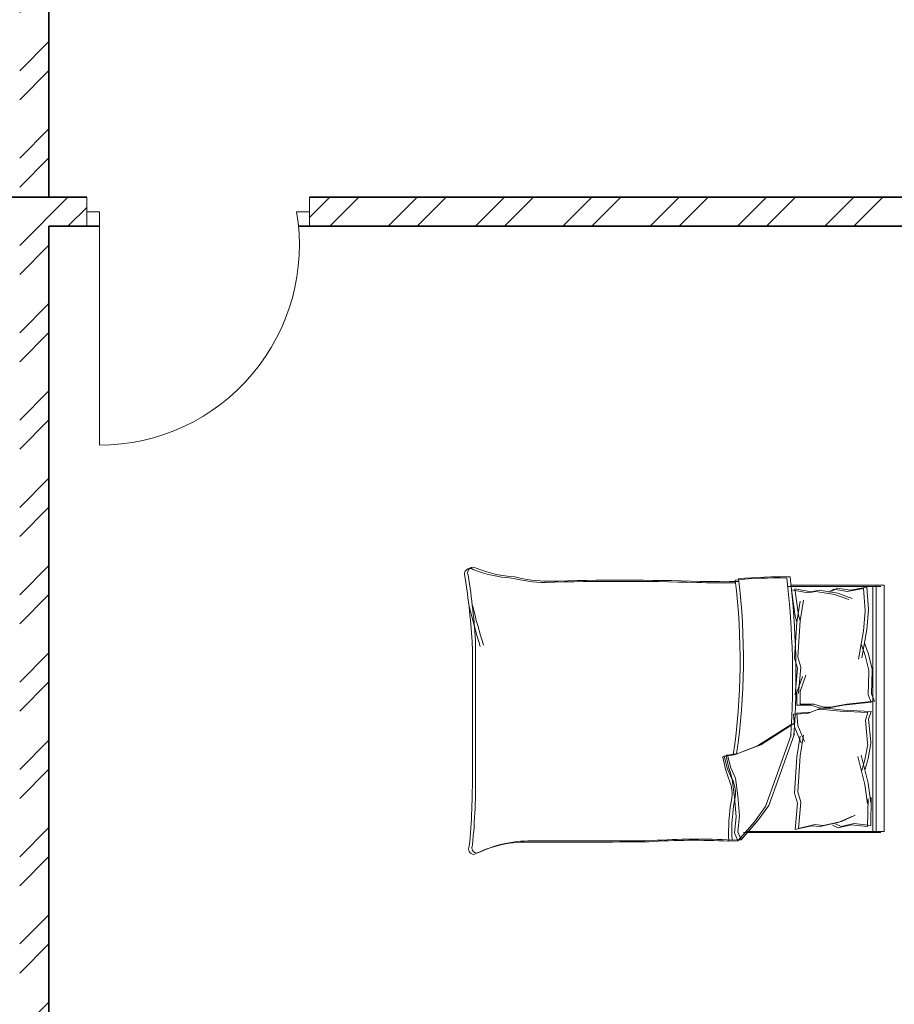
# Model space of a CAD drawing. Units: inches. Extents: x 1962 to 2771, y 1245 to 2660.
# Tile 9 of 114: x 2371 to 2506, y 1527 to 1679. Entities that reach past the tile are written whole.
import ezdxf

# ---------------------------------------------------------------- set-up
doc = ezdxf.new("R2010")
doc.units = ezdxf.units.IN
for name, color, linetype, lineweight in [('A-DOOR', 3, 'Continuous', 18), ('A-FURN', 8, 'Continuous', 13), ('A-WALL', 7, 'Continuous', 35), ('A-WALL-PATT', 252, 'Continuous', 13)]:
    doc.layers.add(name, color=color, linetype=linetype, lineweight=lineweight)

# ---------------------------------------------------------------- blocks, each defined once
blk = doc.blocks.new('BED-PLAN')
for p, q in [((22.05, 42.03), (19.47, 39.08)), ((22.05, 42.02), (19.47, 39.08)), ((22.56, 42.21), (19.98, 39.26)), ((22.56, 42.21), (19.98, 39.26)), ((23.44, 42.09), (22.05, 42.03, 3.08)), ((23.44, 42.09), (22.05, 42.02, 3.08)), ((22.55, 40.8), (22.05, 42.03)), ((22.55, 40.8), (22.05, 42.02)), ((23.95, 42.27), (22.56, 42.21, 3.08)), ((23.95, 42.27), (22.56, 42.21, 3.08)), ((23.06, 40.98), (22.56, 42.21)), ((23.06, 40.98), (22.56, 42.21)), ((0, 40.75), (21.15, 40.75)), ((0, 40.75), (21.15, 40.75)), ((0, 2.76), (0, 40.75)), ((0.51, 40.93), (21.66, 40.93)), ((0.51, 40.93), (21.66, 40.93)), ((1.22, 2.76), (1.22, 40.75)), ((1.22, 2.76), (1.22, 40.75)), ((1.73, 2.95), (1.73, 40.93)), ((1.73, 2.95), (1.73, 40.93)), ((2.03, 39.83), (1.96, 35.54)), ((2.03, 39.83), (1.96, 35.54)), ((2.03, 39.83), (4.58, 39.53)), ((2.03, 39.83), (4.58, 39.53)), ((2.54, 40.02), (2.46, 35.72)), ((2.54, 40.02), (2.46, 35.72)), ((2.54, 40.02), (5.09, 39.72)), ((2.54, 40.02), (5.09, 39.72)), ((4.58, 39.53), (6.63, 40.01)), ((4.58, 39.53), (6.63, 40.01)), ((5.09, 39.72), (7.14, 40.19)), ((5.09, 39.72), (7.14, 40.19)), ((9.4, 39.83), (6.56, 39.2)), ((9.4, 39.83), (6.56, 39.2)), ((6.63, 40.01), (7.46, 39.6)), ((6.63, 40.01), (7.46, 39.6)), ((9.91, 40.02), (7.07, 39.38)), ((9.91, 40.02), (7.07, 39.38)), ((7.14, 40.19), (7.97, 39.78)), ((7.14, 40.19), (7.97, 39.78)), ((10.68, 39.68), (9.4, 39.83)), ((10.68, 39.68), (9.4, 39.83)), ((11.19, 39.87), (9.91, 40.02)), ((11.19, 39.87), (9.91, 40.02)), ((13.17, 40.3), (10.68, 39.68)), ((13.17, 40.3), (10.68, 39.68)), ((13.68, 40.48), (11.19, 39.87)), ((13.68, 40.48), (11.19, 39.87)), ((12.85, 36.22), (13.17, 40.3)), ((12.85, 36.22), (13.17, 40.3)), ((13.36, 36.4), (13.68, 40.48)), ((13.36, 36.4), (13.68, 40.48)), ((22.3, 38.34), (22.55, 40.8)), ((22.3, 38.34), (22.55, 40.8)), ((22.81, 38.52), (23.06, 40.98)), ((22.81, 38.52), (23.06, 40.98)), ((6.56, 39.2), (4.43, 38.26)), ((6.56, 39.2), (4.43, 38.26)), ((7.07, 39.38), (4.94, 38.44)), ((7.07, 39.38), (4.94, 38.44)), ((19.47, 39.08), (17.75, 36.74)), ((19.47, 39.08), (17.75, 36.74)), ((19.98, 39.26), (18.26, 36.92)), ((19.98, 39.26), (18.26, 36.92)), ((22.55, 35.26), (22.3, 38.34)), ((22.55, 35.26), (22.3, 38.34)), ((23.06, 35.45), (22.81, 38.52)), ((23.06, 35.44), (22.81, 38.52)), ((2.46, 35.72), (2.53, 36.52)), ((2.46, 35.72), (2.53, 36.52)), ((2.53, 36.52), (2.95, 33.5)), ((2.53, 36.52), (2.95, 33.5)), ((17.75, 36.74), (16.15, 32.31)), ((17.75, 36.74), (16.15, 32.31)), ((18.26, 36.92), (16.66, 32.49)), ((18.26, 36.92), (16.66, 32.49)), ((1.96, 35.54), (2.02, 36.34)), ((1.96, 35.54), (2.02, 36.34)), ((2.02, 36.34), (2.44, 33.32)), ((2.02, 36.34), (2.44, 33.32)), ((13.3, 34.66), (12.85, 36.22)), ((13.3, 34.66), (12.85, 36.22)), ((13.8, 34.84), (13.36, 36.4)), ((13.8, 34.84), (13.36, 36.4)), ((22.92, 32.56), (22.55, 35.26)), ((22.92, 32.55), (22.55, 35.26)), ((23.42, 32.74), (23.06, 35.45)), ((23.42, 32.74), (23.06, 35.44)), ((2.95, 33.5), (4.02, 29.19)), ((2.95, 33.5), (4.02, 29.19)), ((12.95, 29.09), (13.3, 34.66)), ((12.95, 29.09), (13.3, 34.66)), ((13.46, 29.27), (13.8, 34.84)), ((13.46, 29.27), (13.8, 34.84)), ((2.44, 33.32), (3.52, 29.01)), ((2.44, 33.32), (3.52, 29.01)), ((16.15, 32.31), (13.82, 25.68)), ((16.15, 32.31), (13.82, 25.68)), ((16.66, 32.49), (14.33, 25.86)), ((16.66, 32.49), (14.33, 25.86)), ((23.65, 30.95), (22.92, 32.56)), ((23.65, 30.95), (22.92, 32.55)), ((24.16, 31.14), (23.42, 32.74)), ((24.16, 31.14), (23.42, 32.74)), ((2.92, 31.16), (2.45, 29.52)), ((2.92, 31.16), (2.45, 29.52)), ((3.43, 31.34), (2.96, 29.7)), ((3.43, 31.34), (2.96, 29.7)), ((24.15, 28.99), (23.65, 30.95)), ((24.15, 28.98), (23.65, 30.95)), ((24.65, 29.17), (24.16, 31.14)), ((24.65, 29.17), (24.16, 31.14)), ((62.99, 11.98), (62.99, 31.54)), ((62.99, 11.97), (62.99, 31.54)), ((63.5, 12.16), (63.5, 31.72)), ((63.5, 12.16), (63.5, 31.72)), ((2.45, 29.52), (2.02, 27.19)), ((2.45, 29.52), (2.02, 27.19)), ((2.96, 29.7), (2.52, 27.37)), ((2.96, 29.7), (2.52, 27.37)), ((12.42, 25.89), (12.95, 29.09)), ((12.42, 25.89), (12.95, 29.09)), ((12.93, 26.07), (13.46, 29.27)), ((12.93, 26.07), (13.46, 29.27)), ((19.49, 27.57), (23.06, 28.92)), ((19.49, 27.57), (23.06, 28.92)), ((22.55, 28.74), (24.15, 28.99)), ((22.55, 28.74), (24.15, 28.98)), ((23.06, 28.92), (24.65, 29.17)), ((23.06, 28.92), (24.65, 29.17)), ((2.52, 27.37), (2.54, 27.12)), ((2.52, 27.37), (2.54, 27.12)), ((13.82, 24.05), (18.98, 27.38)), ((13.82, 24.05), (18.98, 27.38)), ((14.33, 24.24), (19.49, 27.57)), ((14.33, 24.24), (19.49, 27.57)), ((18.98, 27.38), (22.55, 28.74)), ((18.98, 27.38), (22.55, 28.74)), ((2.02, 27.19), (2.03, 26.94)), ((2.02, 27.19), (2.03, 26.93)), ((2.03, 26.94), (2.37, 23.42)), ((2.03, 26.93), (2.37, 23.42)), ((2.54, 27.12), (2.88, 23.6)), ((2.54, 27.12), (2.88, 23.6)), ((13.31, 24.44), (12.28, 26.89)), ((13.31, 24.44), (12.28, 26.88)), ((13.81, 24.63), (12.79, 27.07)), ((13.81, 24.63), (12.79, 27.07)), ((13.43, 22.49), (13.31, 24.44)), ((13.43, 22.49), (13.31, 24.44)), ((13.94, 22.68), (13.81, 24.63)), ((13.94, 22.68), (13.81, 24.63)), ((2.37, 23.42), (1.98, 22.24)), ((2.37, 23.42), (1.98, 22.24)), ((2.88, 23.6), (2.49, 22.42)), ((2.88, 23.6), (2.49, 22.42)), ((1.98, 22.24), (6.25, 22.05)), ((1.98, 22.24), (6.25, 22.05)), ((1.99, 20.84), (6.25, 21.3)), ((1.99, 20.84), (6.25, 21.3)), ((2.49, 22.42), (6.76, 22.23)), ((2.49, 22.42), (6.76, 22.23)), ((5.74, 21.11), (8.27, 21.57)), ((5.74, 21.11), (8.27, 21.57)), ((6.25, 22.05), (8.81, 21.75)), ((6.25, 22.05), (8.81, 21.75)), ((6.25, 21.3), (8.78, 21.76)), ((6.25, 21.3), (8.78, 21.76)), ((6.76, 22.23), (9.31, 21.93)), ((6.76, 22.23), (9.31, 21.93)), ((8.27, 21.57), (9.3, 21.57)), ((8.27, 21.57), (9.3, 21.57)), ((8.78, 21.76), (9.81, 21.76)), ((8.78, 21.76), (9.81, 21.76)), ((8.81, 21.75), (9.84, 21.81)), ((8.81, 21.75), (9.84, 21.81)), ((9.3, 21.57), (10.8, 21.11)), ((9.3, 21.57), (10.8, 21.11)), ((9.31, 21.93), (10.35, 21.99)), ((9.31, 21.93), (10.35, 21.99)), ((9.81, 21.76), (11.3, 21.3)), ((9.81, 21.76), (11.3, 21.3)), ((9.84, 21.81), (11.3, 22.36)), ((9.84, 21.81), (11.3, 22.36)), ((10.35, 21.99), (11.81, 22.54)), ((10.35, 21.99), (11.81, 22.54)), ((11.3, 22.36), (13.43, 22.49)), ((11.3, 22.36), (13.43, 22.49)), ((11.3, 21.3), (13.44, 21.3)), ((11.3, 21.3), (13.44, 21.3)), ((11.81, 22.54), (13.94, 22.68)), ((11.81, 22.54), (13.94, 22.68)), ((13.44, 21.3), (13.44, 19.34)), ((13.44, 21.3), (13.44, 19.34)), ((1.49, 20.65), (5.74, 21.11)), ((1.49, 20.65), (5.74, 21.11)), ((1.95, 19.51), (1.49, 20.65)), ((1.95, 19.51), (1.49, 20.65)), ((2.45, 19.69), (1.99, 20.84)), ((2.45, 19.69), (1.99, 20.84)), ((10.8, 21.11), (12.93, 21.11)), ((10.8, 21.11), (12.93, 21.11)), ((12.93, 21.11), (12.93, 19.16)), ((12.93, 21.11), (12.93, 19.16)), ((1.83, 15.97), (1.95, 19.51)), ((1.83, 15.97), (1.95, 19.51)), ((2.34, 16.15), (2.45, 19.69)), ((2.34, 16.15), (2.45, 19.69)), ((12.93, 19.16), (12.06, 16.66)), ((12.93, 19.16), (12.06, 16.66)), ((13.44, 19.34), (12.57, 16.84)), ((13.44, 19.34), (12.57, 16.84)), ((12.85, 15.41), (13.17, 19.49)), ((12.85, 15.41), (13.17, 19.49)), ((13.36, 15.59), (13.68, 19.67)), ((13.36, 15.59), (13.68, 19.67)), ((1.83, 15.72), (1.83, 15.97)), ((1.83, 15.72), (1.83, 15.97)), ((2.41, 13.42), (1.83, 15.72)), ((2.41, 13.42), (1.83, 15.72)), ((2.34, 15.9), (2.34, 16.15)), ((2.34, 15.9), (2.34, 16.15)), ((2.91, 13.6), (2.34, 15.9)), ((2.91, 13.6), (2.34, 15.9)), ((13.3, 13.85), (12.85, 15.41)), ((13.3, 13.85), (12.85, 15.41)), ((13.8, 14.03), (13.36, 15.59)), ((13.8, 14.03), (13.36, 15.59)), ((2.64, 9.63), (3.44, 13.99)), ((2.64, 9.63), (3.44, 13.99)), ((3.14, 9.81), (3.95, 14.17)), ((3.14, 9.81), (3.95, 14.17)), ((12.95, 8.28), (13.3, 13.85)), ((12.95, 8.28), (13.3, 13.85)), ((13.46, 8.46), (13.8, 14.03)), ((13.46, 8.46), (13.8, 14.03)), ((2.98, 11.81), (2.41, 13.42)), ((2.98, 11.81), (2.41, 13.42)), ((3.49, 11.99), (2.91, 13.6)), ((3.49, 11.99), (2.91, 13.6)), ((2.41, 6.59), (2.64, 9.63)), ((2.41, 6.59), (2.64, 9.63)), ((2.91, 6.77), (3.14, 9.81)), ((2.91, 6.77), (3.14, 9.81)), ((12.42, 5.07), (12.95, 8.28)), ((12.42, 5.07), (12.95, 8.28)), ((12.93, 5.26), (13.46, 8.46)), ((12.93, 5.26), (13.46, 8.46)), ((12.95, 8.28), (13.21, 7.38)), ((12.95, 8.28), (13.21, 7.38)), ((13.46, 8.46), (13.72, 7.56)), ((13.46, 8.46), (13.72, 7.56)), ((2.39, 6.5), (2.41, 6.59)), ((2.39, 6.5), (2.41, 6.59)), ((2.65, 3.1), (2.39, 6.5)), ((2.65, 3.1), (2.39, 6.5)), ((2.9, 6.68), (2.91, 6.77)), ((2.9, 6.68), (2.91, 6.77)), ((3.16, 3.28), (2.9, 6.68)), ((3.16, 3.28), (2.9, 6.68)), ((13.21, 7.38), (13.78, 3.33)), ((13.21, 7.38), (13.78, 3.33)), ((13.72, 7.56), (14.29, 3.51)), ((13.72, 7.56), (14.29, 3.51)), ((7.12, 4.02), (4.93, 4.82)), ((7.12, 4.02), (4.93, 4.82)), ((7.63, 4.2), (5.44, 5)), ((7.63, 4.2), (5.44, 5)), ((2.64, 3.1), (5.16, 3.56)), ((2.64, 3.1), (5.16, 3.56)), ((3.14, 3.28), (5.67, 3.74)), ((3.14, 3.28), (5.67, 3.74)), ((5.16, 3.56), (7.23, 3.21)), ((5.16, 3.56), (7.23, 3.21)), ((5.67, 3.74), (7.74, 3.39)), ((5.67, 3.74), (7.74, 3.39)), ((9.99, 3.56), (7.12, 4.02)), ((9.99, 3.56), (7.12, 4.02)), ((7.23, 3.21), (8.04, 3.67)), ((7.23, 3.21), (8.04, 3.67)), ((10.5, 3.74), (7.63, 4.2)), ((10.5, 3.74), (7.63, 4.2)), ((7.74, 3.39), (8.55, 3.85)), ((7.74, 3.39), (8.55, 3.85)), ((11.26, 3.79), (9.99, 3.56)), ((11.26, 3.79), (9.99, 3.56)), ((11.76, 3.97), (10.5, 3.74)), ((11.76, 3.97), (10.5, 3.74)), ((13.78, 3.33), (11.26, 3.79)), ((13.78, 3.33), (11.26, 3.79)), ((14.29, 3.51), (11.76, 3.97)), ((14.29, 3.51), (11.76, 3.97)), ((14.4, 2.76), (0, 2.76)), ((14.4, 2.76), (0, 2.76)), ((14.9, 2.95), (0.51, 2.95)), ((14.9, 2.95), (0.51, 2.95))]:
    blk.add_line(p, q)
for centre, radius, start, end in [((54.58, 60.54), 18.33, 267.4714, 296.4681), ((54.58, 60.54), 18.33, 267.4714, 296.4681), ((55.09, 60.72), 18.33, 267.4714, 296.4681), ((55.09, 60.72), 18.33, 267.4714, 296.4681), ((62.69, 43.25), 0.876, 332.6588, 86.02), ((62.69, 43.25), 0.876, 332.6588, 86.02), ((63.2, 43.43), 0.876, 332.6588, 86.02), ((63.2, 43.43), 0.876, 332.6588, 86.02), ((168.74, 32.71), 105.75, 174.4998, 180.6351), ((168.74, 32.71), 105.75, 174.4998, 180.6351), ((169.24, 32.89), 105.75, 174.4998, 180.6351), ((169.24, 32.89), 105.75, 174.4998, 180.6351), ((-5.29, 40.8), 28.76, 349.8763, 2.5657), ((-5.29, 40.8), 28.76, 349.8763, 2.5657), ((28.87, 144.88), 102.94, 266.9791, 273.8365), ((28.87, 144.88), 102.94, 266.9791, 273.8365), ((-4.78, 40.98), 28.76, 349.8763, 2.5657), ((-4.78, 40.98), 28.76, 349.8763, 2.5657), ((29.37, 145.06), 102.94, 266.9791, 273.8365), ((29.37, 145.06), 102.94, 266.9791, 273.8365), ((53.91, -3583.94), 3626.16, 90.00217, 90.28689), ((53.91, -3583.94), 3626.16, 90.00217, 90.28689), ((54.42, -3583.75), 3626.16, 90.00217, 90.28689), ((54.42, -3583.75), 3626.16, 90.00217, 90.28689), ((27.87, 34.77), 4.95, 168.6608, 203.7384), ((27.87, 34.77), 4.95, 168.6608, 203.7384), ((28.38, 34.95), 4.95, 168.6608, 203.7384), ((28.38, 34.95), 4.95, 168.6608, 203.7384), ((1.18, 24.77), 23.57, 10.6617, 19.8806), ((1.18, 24.76), 23.57, 10.6617, 19.8806), ((1.69, 24.95), 23.57, 10.6617, 19.8806), ((1.69, 24.95), 23.57, 10.6617, 19.8806), ((124.76, 14.3), 102.56, 171.7845, 186.9006), ((124.76, 14.3), 102.56, 171.7845, 186.9006), ((24.2, 29.12), 0.147, 250.2464, 1.1377), ((24.2, 29.12), 0.147, 250.2464, 1.1377), ((24.7, 29.3), 0.147, 250.2464, 1.1377), ((24.7, 29.3), 0.147, 250.2464, 1.1377), ((124.25, 14.12), 102.56, 171.7845, 186.9006), ((124.25, 14.11), 102.56, 171.7845, 186.9006), ((144.71, 16.98), 131.13, 176.0865, 186.7821), ((144.71, 16.98), 131.13, 176.0865, 186.7821), ((145.22, 17.16), 131.13, 176.0865, 186.7821), ((145.22, 17.16), 131.13, 176.0865, 186.7821), ((-18.34, -13.51), 84.62, 13.3832, 17.7053), ((-18.34, -13.51), 84.62, 13.3832, 17.7053), ((160.15, 17.21), 96.78, 182.9958, 189.4091), ((160.15, 17.21), 96.78, 182.9958, 189.4091), ((-18.85, -13.69), 84.62, 13.3832, 17.7053), ((-18.85, -13.69), 84.62, 13.3832, 17.7053), ((159.64, 17.03), 96.78, 182.9958, 189.4091), ((159.64, 17.03), 96.78, 182.9958, 189.4091), ((15.97, 67.7), 66.22, 268.7218, 275.604), ((15.97, 67.7), 66.22, 268.7218, 275.604), ((16.48, 67.88), 66.22, 268.7218, 275.604), ((16.48, 67.88), 66.22, 268.7218, 275.604), ((24.78, -132.99), 135.22, 88.4762, 91.0082), ((24.78, -132.99), 135.22, 88.4762, 91.0082), ((25.29, -132.81), 135.22, 88.4762, 91.0082), ((25.29, -132.81), 135.22, 88.4762, 91.0082), ((40.23, 385.38), 383.38, 268.2277, 271.7185), ((40.23, 385.38), 383.38, 268.2277, 271.7185), ((40.74, 385.56), 383.38, 268.2277, 271.7185), ((40.74, 385.56), 383.38, 268.2277, 271.7185), ((51.28, -21.38), 23.56, 76.0648, 88.9113), ((51.28, -21.38), 23.56, 76.0648, 88.9113), ((51.79, -21.2), 23.56, 76.0648, 88.9113), ((51.79, -21.2), 23.56, 76.0648, 88.9113), ((56.37, -17.03), 18.73, 67.9751, 86.652), ((56.37, -17.03), 18.73, 67.9751, 86.652), ((55.86, -17.22), 18.73, 67.9751, 86.652), ((55.86, -17.22), 18.73, 67.9751, 86.652), ((63.37, 0.87), 0.866, 236.1736, 23.4781), ((63.37, 0.87), 0.866, 236.1736, 23.4781), ((63.87, 1.05), 0.866, 236.1736, 23.4781), ((63.87, 1.05), 0.866, 236.1736, 23.4781)]:
    blk.add_arc(centre, radius, start, end)

msp = doc.modelspace()

# ---------------------------------------------------------------- hatches: boundary and pattern name
at = {"layer": 'A-WALL-PATT'}
h = msp.add_hatch(dxfattribs=at)
h.set_pattern_fill('ANSI32', color=256)
h.paths.add_polyline_path([(2090.8074, 2467.3437), (2141.6481, 2467.3437), (2141.6481, 2469.5937), (2141.6481, 2471.8437), (2086.3074, 2471.8437), (2086.3074, 2422.5333), (2090.8074, 2422.5333)])
h.paths.add_polyline_path([(2282.7664, 2471.8437), (2204.8982, 2471.8437), (2204.8982, 2467.3437), (2234.8074, 2467.3437), (2234.8074, 2311.3437), (2228.7492, 2311.3437), (2228.7492, 2306.8437), (2234.8074, 2306.8437), (2331.9227, 2306.8437), (2331.9227, 2309.0937), (2331.9227, 2311.3437), (2239.3074, 2311.3437), (2239.3074, 2467.3437), (2282.7664, 2467.3437), (2282.7664, 2469.5937)])
h.paths.add_polyline_path([(2471.4531, 2519.8437), (2552.011, 2519.8437), (2564.3996, 2519.8437), (2564.3996, 2511.1389), (2568.8996, 2511.1389), (2568.8996, 2524.3437), (2466.9531, 2524.3437), (2466.9531, 2471.8437), (2450.0749, 2471.8437), (2446.4672, 2471.8437), (2446.4672, 2467.3437), (2450.0749, 2467.3437), (2475.9988, 2467.3437), (2475.9988, 2469.5937), (2475.9988, 2471.8437), (2471.4531, 2471.8437)])
h.paths.add_polyline_path([(2575.2231, 2469.5937), (2575.2231, 2471.8437), (2568.8996, 2471.8437), (2568.8996, 2487.1389), (2564.3996, 2487.1389), (2564.3996, 2471.8437), (2556.511, 2471.8437), (2499.2904, 2471.8437), (2499.2904, 2467.3437), (2507.8074, 2467.3437), (2507.8074, 2311.3437), (2414.863, 2311.3437), (2414.863, 2306.8437), (2512.3074, 2306.8437), (2517.0114, 2306.8437), (2517.0114, 2309.0937), (2517.0114, 2311.3437), (2512.3074, 2311.3437), (2512.3074, 2467.3437), (2575.2231, 2467.3437)])
h.paths.add_polyline_path([(2660.8074, 2471.8437), (2600.9602, 2471.8437), (2600.9602, 2467.3437), (2656.3074, 2467.3437), (2656.3074, 2432.5704), (2660.8074, 2432.5704)])
h.paths.add_polyline_path([(2660.8074, 2372.5704), (2656.3074, 2372.5704), (2656.3074, 2311.3437), (2600.276, 2311.3437), (2600.276, 2309.0937), (2600.276, 2306.8437), (2656.3074, 2306.8437), (2656.3074, 2296.2593), (2660.8074, 2296.2593)])
h.paths.add_polyline_path([(2572.3074, 2306.8437), (2577.1385, 2306.8437), (2577.1385, 2311.3437), (2551.082, 2311.3437), (2551.082, 2306.8437), (2567.8074, 2306.8437), (2567.8074, 2258.8437), (2540.0574, 2258.8437), (2540.0574, 2256.5937), (2540.0574, 2254.3437), (2567.8074, 2254.3437), (2656.3074, 2254.3437), (2656.3074, 2236.9085), (2660.8074, 2236.9085), (2660.8074, 2272.2593), (2656.3074, 2272.2593), (2656.3074, 2258.8437), (2572.3074, 2258.8437)])
h.paths.add_polyline_path([(2512.3074, 2254.3437), (2518.8716, 2254.3437), (2518.8716, 2256.5937), (2518.8716, 2258.8437), (2507.8074, 2258.8437), (2507.8074, 2177.8437), (2567.8074, 2177.8437), (2567.8074, 2172.9628), (2572.3074, 2172.9628), (2572.3074, 2177.8437), (2656.3074, 2177.8437), (2656.3074, 2166.4846), (2660.8074, 2166.4846), (2660.8074, 2200.9085), (2656.3074, 2200.9085), (2656.3074, 2182.3437), (2512.3074, 2182.3437)])
h.paths.add_polyline_path([(2656.3074, 2129.8437), (2572.3074, 2129.8437), (2572.3074, 2150.3044), (2570.0574, 2150.3044), (2567.8074, 2150.3044), (2567.8074, 2129.8437), (2507.8074, 2129.8437), (2507.8074, 2116.3027), (2510.0574, 2116.3027), (2512.3074, 2116.3027), (2512.3074, 2125.3437), (2567.8074, 2125.3437), (2572.3074, 2125.3437), (2656.3074, 2125.3437)])
h.paths.add_polyline_path([(2090.8074, 2362.5333), (2086.3074, 2362.5333), (2086.3074, 2298.6242), (2090.8074, 2298.6242), (2090.8074, 2306.8437), (2174.8074, 2306.8437), (2174.8074, 2286.4178), (2179.3074, 2286.4178), (2179.3074, 2306.8437), (2192.8641, 2306.8437), (2192.8641, 2309.0937), (2192.8641, 2311.3437), (2090.8074, 2311.3437)])
h.paths.add_polyline_path([(2209.156, 2258.8437), (2179.3074, 2258.8437), (2179.3074, 2263.2236), (2177.0574, 2263.2236), (2174.8074, 2263.2236), (2174.8074, 2258.8437), (2090.8074, 2258.8437), (2090.8074, 2274.6242), (2086.3074, 2274.6242), (2086.3074, 2238.2967), (2088.5574, 2238.2967), (2090.8074, 2238.2967), (2090.8074, 2254.3437), (2209.156, 2254.3437)])
h.paths.add_polyline_path([(2090.8074, 2177.8437), (2234.8074, 2177.8437), (2234.8074, 2173.1428), (2239.3074, 2173.1428), (2239.3074, 2258.8437), (2230.8442, 2258.8437), (2230.8442, 2256.5937), (2230.8442, 2254.3437), (2234.8074, 2254.3437), (2234.8074, 2182.3437), (2090.8074, 2182.3437), (2090.8074, 2202.2967), (2086.3074, 2202.2967), (2086.3074, 2140.0389), (2090.8074, 2140.0389)])
h.paths.add_polyline_path([(2090.8074, 2080.0389), (2086.3074, 2080.0389), (2086.3074, 2033.8437), (2090.8074, 2033.8437)], flags=17)
h.paths.add_polyline_path([(2244.9405, 2033.8437), (2239.3074, 2033.8437), (2239.3074, 2142.0665), (2237.2592, 2142.0665), (2234.8074, 2142.0665), (2234.8074, 2033.8437), (2090.8074, 2033.8437), (2076.5204, 2033.8437), (2072.0204, 2033.8437), (2072.0204, 2000.4493), (2076.5204, 2000.4493), (2076.5204, 2029.3437), (2090.8074, 2029.3437), (2244.9405, 2029.3437), (2244.9405, 2031.5937)])
h.paths.add_polyline_path([(2234.8074, 1933.3437), (2076.5204, 1933.3437), (2076.5204, 1952.4493), (2074.2704, 1952.4493), (2072.0204, 1952.4493), (2072.0204, 1933.3437), (2072.0204, 1928.8437), (2234.8074, 1928.8437)])
h.paths.add_polyline_path([(2090.8074, 1928.8437), (2086.3074, 1928.8437), (2086.3074, 1906.5013), (2090.8074, 1906.5013)])
h.paths.add_polyline_path([(2090.8074, 1846.5013), (2086.3074, 1846.5013), (2086.3074, 1769.9917), (2088.5574, 1769.9917), (2090.8074, 1769.9917), (2090.8074, 1780.3437), (2234.8074, 1780.3437), (2234.8074, 1708.3437), (2230.3764, 1708.3437), (2230.3764, 1703.8437), (2239.3074, 1703.8437), (2239.3074, 1792.6669), (2237.0574, 1792.6669), (2234.8074, 1792.6669), (2234.8074, 1784.8437), (2090.8074, 1784.8437)])
h.paths.add_polyline_path([(2239.3074, 1928.8437), (2244.9405, 1928.8437), (2244.9405, 1931.0937), (2244.9405, 1933.3437), (2234.8074, 1933.3437), (2234.8074, 1928.8437), (2234.8074, 1825.5949), (2239.3074, 1825.5949)])
h.paths.add_polyline_path([(2148.0425, 1649.0937), (2148.0425, 1651.3437), (2090.8074, 1651.3437), (2090.8074, 1646.8437), (2148.0425, 1646.8437)], flags=0)
h.paths.add_polyline_path([(2207.5601, 1708.3437), (2090.8074, 1708.3437), (2090.8074, 1703.8437), (2174.8074, 1703.8437), (2174.8074, 1651.3437), (2170.4457, 1651.3437), (2170.4457, 1646.8437), (2195.9924, 1646.8437), (2195.9924, 1649.0937), (2195.9924, 1651.3437), (2179.3074, 1651.3437), (2179.3074, 1703.8437), (2207.5601, 1703.8437), (2207.5601, 1706.0937)])
h.paths.add_polyline_path([(2090.8074, 1733.9917), (2086.3074, 1733.9917), (2086.3074, 1696.1032), (2088.5574, 1696.1032), (2090.8074, 1696.1032)])
h.paths.add_polyline_path([(2090.8074, 1672.1032), (2086.3074, 1672.1032), (2086.3074, 1600.3335), (2090.8074, 1600.3335)])
h.paths.add_polyline_path([(2090.8074, 1540.3335), (2086.3074, 1540.3335), (2086.3074, 1486.3437), (2139.6766, 1486.3437), (2139.6766, 1490.8437), (2090.8074, 1490.8437)])
h.paths.add_polyline_path([(2302.3876, 1490.8437), (2239.3074, 1490.8437), (2239.3074, 1646.8437), (2335.9994, 1646.8437), (2335.9994, 1651.3437), (2229.884, 1651.3437), (2229.884, 1646.8437), (2234.8074, 1646.8437), (2234.8074, 1490.8437), (2202.7103, 1490.8437), (2202.7103, 1488.5937), (2202.7103, 1486.3437), (2275.0699, 1486.3437), (2275.0699, 1475.772), (2279.5699, 1475.772), (2279.5699, 1486.3437), (2302.3876, 1486.3437)])
h.paths.add_polyline_path([(2279.5699, 1451.772), (2275.0699, 1451.772), (2275.0699, 1438.3437), (2174.8074, 1438.3437), (2174.8074, 1486.3437), (2179.7922, 1486.3437), (2179.7922, 1490.8437), (2163.3585, 1490.8437), (2163.3585, 1488.5937), (2163.3585, 1486.3437), (2170.3074, 1486.3437), (2170.3074, 1433.8437), (2279.5699, 1433.8437)])
h.paths.add_polyline_path([(2427.2363, 1490.8437), (2375.8074, 1490.8437), (2375.8074, 1646.8437), (2381.6401, 1646.8437), (2381.6401, 1651.3437), (2365.887, 1651.3437), (2365.887, 1649.0937), (2365.887, 1646.8437), (2371.3074, 1646.8437), (2371.3074, 1490.8437), (2327.5627, 1490.8437), (2327.5627, 1488.5937), (2327.5627, 1486.3437), (2371.3074, 1486.3437), (2371.3074, 1433.8437), (2375.8074, 1433.8437), (2375.8074, 1486.3437), (2427.2363, 1486.3437)])
h.paths.add_polyline_path([(2512.3074, 1646.8437), (2519.4351, 1646.8437), (2519.4351, 1649.0937), (2519.4351, 1651.3437), (2507.8074, 1651.3437), (2416.0063, 1651.3437), (2416.0063, 1649.0937), (2416.0063, 1646.8437), (2507.8074, 1646.8437), (2507.8074, 1490.8437), (2497.0532, 1490.8437), (2497.0532, 1488.5937), (2497.0532, 1486.3437), (2574.9344, 1486.3437), (2574.9344, 1476.0181), (2579.4344, 1476.0181), (2579.4344, 1486.3437), (2584.4872, 1486.3437), (2584.3074, 1490.8437), (2512.3074, 1490.8437)])
h.paths.add_polyline_path([(2470.5091, 1486.3437), (2473.9767, 1486.3437), (2473.9767, 1490.8437), (2449.6605, 1490.8437), (2449.6605, 1488.5937), (2449.6605, 1486.3437), (2466.0091, 1486.3437), (2466.0091, 1433.8437), (2470.5091, 1433.8437), (2579.4344, 1433.8437), (2579.4344, 1452.0181), (2574.9344, 1452.0181), (2574.9344, 1438.3437), (2554.5091, 1438.3437), (2470.5091, 1438.3437)])
h.paths.add_polyline_path([(2656.3074, 1490.8437), (2611.86, 1490.8437), (2611.86, 1486.3437), (2656.3074, 1486.3437)])
h.paths.add_polyline_path([(2660.8074, 1532.7007), (2658.5574, 1532.7007), (2656.3074, 1532.7007), (2656.3074, 1486.3437), (2660.8074, 1486.3437)])
h.paths.add_polyline_path([(2660.8074, 1664.9663), (2656.3074, 1664.9663), (2656.3074, 1651.3437), (2602.2313, 1651.3437), (2602.2313, 1646.8437), (2656.3074, 1646.8437), (2656.3074, 1592.7007), (2660.8074, 1592.7007)])
h.paths.add_polyline_path([(2660.8074, 1724.5221), (2656.3074, 1724.5221), (2656.3074, 1703.8437), (2542.4725, 1703.8437), (2542.4725, 1699.3437), (2567.8074, 1699.3437), (2567.8074, 1651.3437), (2552.7766, 1651.3437), (2552.7766, 1649.0937), (2552.7766, 1646.8437), (2577.2878, 1646.8437), (2577.2878, 1649.0937), (2577.2878, 1651.3437), (2572.3074, 1651.3437), (2572.3074, 1699.3437), (2656.3074, 1699.3437), (2656.3074, 1688.9663), (2660.8074, 1688.9663)])
h.paths.add_polyline_path([(2660.8074, 1880.6524), (2656.3074, 1880.6524), (2656.3074, 1832.8437), (2512.3074, 1832.8437), (2512.3074, 1837.8959), (2507.8074, 1837.8959), (2507.8074, 1828.3437), (2567.8074, 1828.3437), (2567.8074, 1804.3437), (2572.3074, 1804.3437), (2572.3074, 1828.3437), (2656.3074, 1828.3437), (2656.3074, 1818.6778), (2660.8074, 1818.6778)])
h.paths.add_polyline_path([(2660.8074, 1794.6778), (2656.3074, 1794.6778), (2656.3074, 1780.3437), (2572.3074, 1780.3437), (2572.3074, 1783.0303), (2570.0574, 1783.0303), (2567.8074, 1783.0303), (2567.8074, 1780.3437), (2507.8074, 1780.3437), (2507.8074, 1699.3437), (2517.8858, 1699.3437), (2517.8858, 1701.5937), (2517.8858, 1703.8437), (2512.3074, 1703.8437), (2512.3074, 1775.8437), (2656.3074, 1775.8437), (2656.3074, 1760.5221), (2660.8074, 1760.5221)])
h.paths.add_polyline_path([(2660.8074, 1981.3437), (2660.8074, 2020.2808), (2658.5574, 2020.2808), (2656.3074, 2020.2808), (2656.3074, 1981.3437), (2512.3074, 1981.3437), (2512.3074, 2086.6996), (2507.8074, 2086.6996), (2507.8074, 1981.3437), (2375.8074, 1981.3437), (2375.8074, 1986.8505), (2373.5574, 1986.8505), (2371.3074, 1986.8505), (2371.3074, 1973.2607), (2375.8074, 1973.2607), (2375.8074, 1976.8437), (2507.8074, 1976.8437), (2507.8074, 1865.4281), (2510.0574, 1865.4281), (2512.3074, 1865.4281), (2512.3074, 1976.8437), (2660.8074, 1976.8437)])
h.paths.add_polyline_path([(2375.8074, 1940.297), (2373.5574, 1940.297), (2371.3074, 1940.297), (2371.3074, 1933.3437), (2278.4434, 1933.3437), (2278.4434, 1928.8437), (2371.3074, 1928.8437), (2371.3074, 1651.3437), (2375.8074, 1651.3437)])
h.paths.add_polyline_path([(2660.8074, 1976.8437), (2656.3074, 1976.8437), (2656.3074, 1940.6524), (2660.8074, 1940.6524)], flags=17)
h.paths.add_polyline_path([(2660.8074, 2142.4846), (2656.3074, 2142.4846), (2656.3074, 2080.2808), (2660.8074, 2080.2808)])
h.paths.add_polyline_path([(2381.4189, 2311.3437), (2375.8074, 2311.3437), (2375.8074, 2467.3437), (2424.7242, 2467.3437), (2424.7242, 2469.5937), (2424.7242, 2471.8437), (2375.8074, 2471.8437), (2375.8074, 2524.3437), (2371.3074, 2524.3437), (2371.3074, 2471.8437), (2307.2097, 2471.8437), (2307.2097, 2467.3437), (2371.3074, 2467.3437), (2371.3074, 2311.3437), (2366.8901, 2311.3437), (2366.8901, 2306.8437), (2371.3074, 2306.8437), (2371.3074, 2033.8437), (2279.6589, 2033.8437), (2279.6589, 2029.3437), (2371.3074, 2029.3437), (2371.3074, 2014.2598), (2375.8074, 2014.2598), (2375.8074, 2306.8437), (2381.4189, 2306.8437)])
h.paths.add_polyline_path([(2263.3074, 2524.3437), (2170.3074, 2524.3437), (2170.3074, 2519.8437), (2170.3074, 2471.8437), (2165.0312, 2471.8437), (2165.0312, 2467.3437), (2179.6721, 2467.3437), (2179.6721, 2469.5161), (2179.6721, 2471.8437), (2174.8074, 2471.8437), (2174.8074, 2519.8437), (2258.8074, 2519.8437), (2258.8074, 2511.6436), (2263.3074, 2511.6436)])
h.paths.add_polyline_path([(2245.0232, 1361.4123), (2492.9468, 1361.4123), (2492.9468, 1398.505), (2245.0232, 1398.505)], flags=9)
h.paths.add_polyline_path([(2388.1434, 2086.6936), (2425.0704, 2086.6936), (2425.0704, 2105.3509), (2388.1434, 2105.3509)], flags=9)
h.paths.add_polyline_path([(2404.922, 2242.6744), (2445.7337, 2242.6744), (2445.7337, 2261.3318), (2404.922, 2261.3318)], flags=9)
h.paths.add_polyline_path([(2269.4107, 2156.7935), (2306.3378, 2156.7935), (2306.3378, 2175.4508), (2269.4107, 2175.4508)], flags=9)
h.paths.add_polyline_path([(2269.3277, 2233.4343), (2306.2547, 2233.4343), (2306.2547, 2252.0917), (2269.3277, 2252.0917)], flags=9)
h.paths.add_polyline_path([(2431.6052, 2320.6922), (2470.4456, 2320.6922), (2470.4456, 2339.3495), (2431.6052, 2339.3495)], flags=25)
h.paths.add_polyline_path([(2249.6902, 2315.7608), (2288.5306, 2315.7608), (2288.5306, 2334.4182), (2249.6902, 2334.4182)], flags=25)
h.paths.add_polyline_path([(2096.9301, 2314.3181), (2135.7704, 2314.3181), (2135.7704, 2332.9755), (2096.9301, 2332.9755)], flags=25)
h.paths.add_polyline_path([(2134.3475, 2285.7089), (2161.4655, 2285.7089), (2161.4655, 2304.3662), (2134.3475, 2304.3662)], flags=9)
h.paths.add_polyline_path([(2126.5155, 2209.4076), (2159.9227, 2209.4076), (2159.9227, 2228.065), (2126.5155, 2228.065)], flags=25)
h.paths.add_polyline_path([(2110.5753, 2141.5299), (2149.4157, 2141.5299), (2149.4157, 2160.1872), (2110.5753, 2160.1872)], flags=25)
h.paths.add_polyline_path([(2249.8618, 1968.3317), (2286.3966, 1968.3317), (2286.3966, 1986.989), (2249.8618, 1986.989)], flags=9)
h.paths.add_polyline_path([(2395.9507, 1777.0051), (2436.7624, 1777.0051), (2436.7624, 1795.6625), (2395.9507, 1795.6625)], flags=9)
h.paths.add_polyline_path([(2398.5259, 1888.5651), (2435.0062, 1888.5651), (2435.0062, 1907.2224), (2398.5259, 1907.2224)], flags=25)
h.paths.add_polyline_path([(2259.3506, 1728.3559), (2296.2776, 1728.3559), (2296.2776, 1747.0132), (2259.3506, 1747.0132)], flags=9)
h.paths.add_polyline_path([(2271.3698, 1845.268), (2308.2968, 1845.268), (2308.2968, 1863.9253), (2271.3698, 1863.9253)], flags=9)
h.paths.add_polyline_path([(2120.9355, 1786.3027), (2159.7759, 1786.3027), (2159.7759, 1804.9601), (2120.9355, 1804.9601)], flags=25)
h.paths.add_polyline_path([(2121.3164, 1732.1043), (2154.7236, 1732.1043), (2154.7236, 1750.7616), (2121.3164, 1750.7616)], flags=25)
h.paths.add_polyline_path([(2118.3706, 1678.8997), (2147.5282, 1678.8997), (2147.5282, 1697.557), (2118.3706, 1697.557)], flags=25)
h.paths.add_polyline_path([(2385.9227, 1493.557), (2424.763, 1493.557), (2424.763, 1512.2143), (2385.9227, 1512.2143)], flags=25)
h.paths.add_polyline_path([(2248.7058, 1500.0256), (2287.5462, 1500.0256), (2287.5462, 1518.6829), (2248.7058, 1518.6829)], flags=25)
h.paths.add_polyline_path([(2104.1669, 1617.3771), (2143.0073, 1617.3771), (2143.0073, 1636.0344), (2104.1669, 1636.0344)], flags=9)
h.paths.add_polyline_path([(2096.0714, 1447.8824), (2137.3845, 1447.8824), (2137.3845, 1458.1859), (2096.0714, 1458.1859)], flags=9)
h.paths.add_polyline_path([(2180.6114, 1440.325), (2209.7689, 1440.325), (2209.7689, 1458.9823), (2180.6114, 1458.9823)], flags=25)
h.paths.add_polyline_path([(2316.1698, 1447.9637), (2357.4829, 1447.9637), (2357.4829, 1458.2673), (2316.1698, 1458.2673)], flags=9)
h.paths.add_polyline_path([(2397.6187, 1447.9637), (2438.9318, 1447.9637), (2438.9318, 1458.2673), (2397.6187, 1458.2673)], flags=9)
h.paths.add_polyline_path([(2473.0778, 1439.5953), (2502.2354, 1439.5953), (2502.2354, 1458.2527), (2473.0778, 1458.2527)], flags=25)
h.paths.add_polyline_path([(2589.7027, 1447.8819), (2631.0158, 1447.8819), (2631.0158, 1458.1855), (2589.7027, 1458.1855)], flags=9)
h.paths.add_polyline_path([(2522.4009, 1497.5285), (2561.2413, 1497.5285), (2561.2413, 1516.1859), (2522.4009, 1516.1859)], flags=25)
h.paths.add_polyline_path([(2579.6565, 1671.3482), (2608.8141, 1671.3482), (2608.8141, 1690.0056), (2579.6565, 1690.0056)], flags=25)
h.paths.add_polyline_path([(2544.7038, 1725.5064), (2578.1111, 1725.5064), (2578.1111, 1744.1637), (2544.7038, 1744.1637)], flags=25)
h.paths.add_polyline_path([(2578.1191, 1807.472), (2607.2766, 1807.472), (2607.2766, 1826.1293), (2578.1191, 1826.1293)], flags=25)
h.paths.add_polyline_path([(2595.0614, 1835.1839), (2633.9018, 1835.1839), (2633.9018, 1853.8413), (2595.0614, 1853.8413)], flags=25)
h.paths.add_polyline_path([(2567.0097, 2097.7035), (2605.8501, 2097.7035), (2605.8501, 2116.3609), (2567.0097, 2116.3609)], flags=9)
h.paths.add_polyline_path([(2586.644, 2134.6454), (2615.8015, 2134.6454), (2615.8015, 2153.3027), (2586.644, 2153.3027)], flags=9)
h.paths.add_polyline_path([(2544.6185, 2212.6783), (2578.0258, 2212.6783), (2578.0258, 2231.3356), (2544.6185, 2231.3356)], flags=25)
h.paths.add_polyline_path([(2577.0273, 2256.9023), (2606.1849, 2256.9023), (2606.1849, 2275.5597), (2577.0273, 2275.5597)], flags=24)
h.paths.add_polyline_path([(2605.2683, 2315.2821), (2644.1087, 2315.2821), (2644.1087, 2333.9395), (2605.2683, 2333.9395)], flags=25)
h.paths.add_polyline_path([(2583.1244, 2496.1815), (2624.4375, 2496.1815), (2624.4375, 2506.4851), (2583.1244, 2506.4851)], flags=9)
h.paths.add_polyline_path([(2474.761, 2497.0823), (2503.9185, 2497.0823), (2503.9185, 2515.7397), (2474.761, 2515.7397)], flags=25)
h.paths.add_polyline_path([(2387.5787, 2494.2563), (2428.902, 2494.2563), (2428.902, 2504.5598), (2387.5787, 2504.5598)], flags=9)
h.paths.add_polyline_path([(2300.1657, 2500.1564), (2341.4788, 2500.1564), (2341.4788, 2510.46), (2300.1657, 2510.46)], flags=25)
h.paths.add_polyline_path([(2176.8589, 2497.5843), (2206.0165, 2497.5843), (2206.0165, 2516.2416), (2176.8589, 2516.2416)], flags=25)
h.paths.add_polyline_path([(2097.4668, 2494.9762), (2138.7799, 2494.9762), (2138.7799, 2505.2798), (2097.4668, 2505.2798)], flags=9)

# ---------------------------------------------------------------- linework, layer by layer
at = {"layer": 'A-DOOR'}
for p, q in [((2381.6401, 1646.8437), (2381.6401, 1651.3437)), ((2381.6401, 1651.3437), (2381.6401, 1649.0937)), ((2416.0063, 1646.8437), (2416.0063, 1651.3437)), ((2416.0063, 1651.3437), (2416.0063, 1649.0937)), ((2381.6401, 1649.0937), (2383.6401, 1649.0937)), ((2383.6401, 1649.0937), (2383.6401, 1613.0937)), ((2416.0063, 1649.0937), (2414.0063, 1649.0937))]:
    msp.add_line(p, q, dxfattribs=at)
msp.add_arc((2383.6401, 1643.9007), 30.807, 270, 9.704382, dxfattribs=at)
at = {"layer": 'A-WALL'}
for p, q in [((2375.8074, 1941.894), (2375.8074, 1651.3437)), ((2381.6401, 1651.3437), (2365.887, 1651.3437)), ((2507.8074, 1651.3437), (2416.0063, 1651.3437)), ((2375.8074, 1646.8437), (2375.8074, 1490.8437)), ((2383.6401, 1646.8437), (2375.8074, 1646.8437)), ((2507.8074, 1646.8437), (2414.3062, 1646.8437))]:
    msp.add_line(p, q, dxfattribs=at)

# ---------------------------------------------------------------- block references
at = {"layer": 'A-FURN', "rotation": 180}
msp.add_blockref('BED-PLAN', (2504.6288, 1594.262), dxfattribs=at)

doc.saveas('drawing.dxf')
